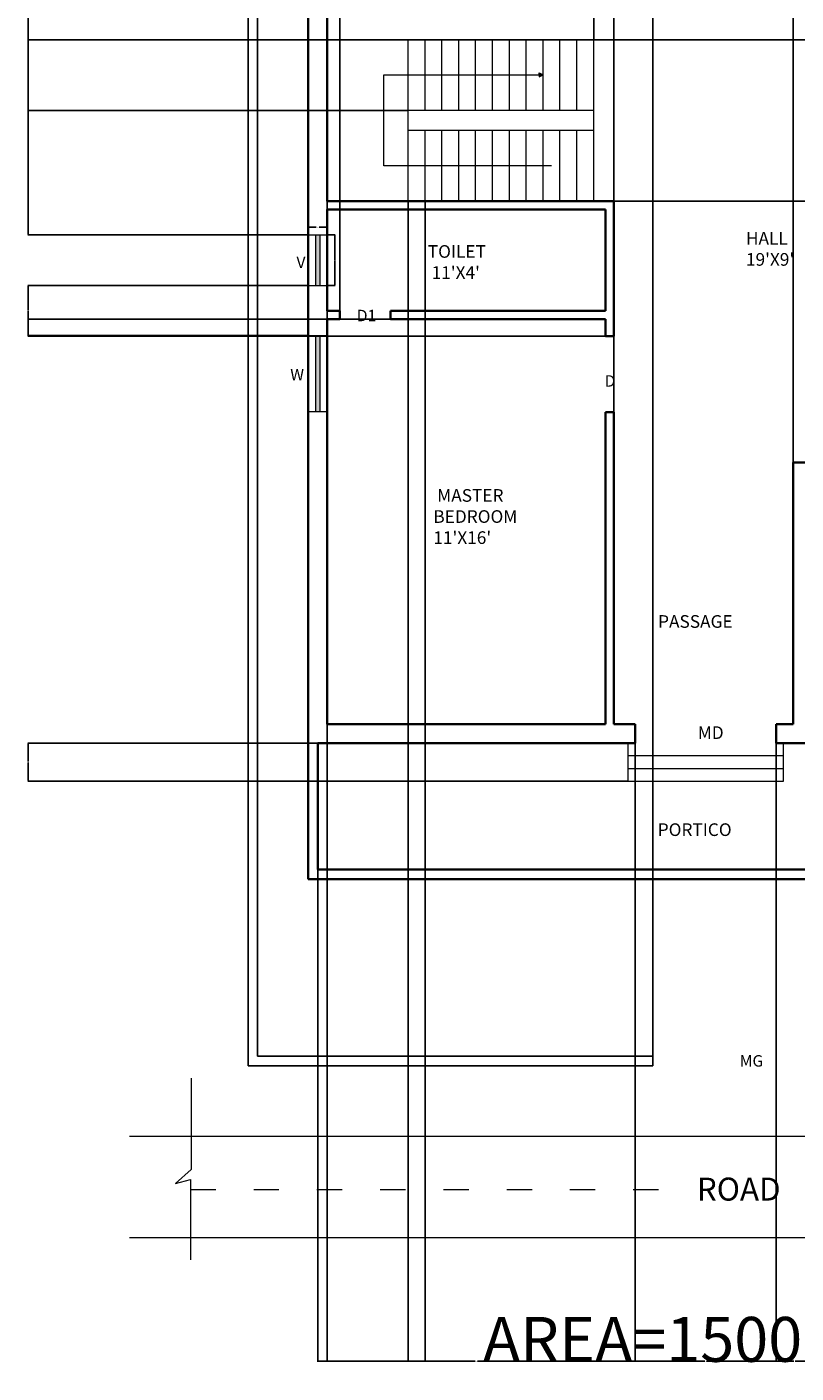
# Model space of a CAD drawing. Units: inches. Extents: x 502 to 1235, y -850 to 110.
# Tile 1 of 9: x 502 to 867, y -850 to -212. Entities that reach past the tile are written whole.
import ezdxf

# ---------------------------------------------------------------- set-up
doc = ezdxf.new("R2010")
doc.units = ezdxf.units.IN
doc.header["$MEASUREMENT"] = 0
doc.linetypes.add('ACAD_ISO03W100', pattern=[30, 12, -18])
for name, color, linetype, lineweight in [('A-ANNO-DIMS', 2, 'Continuous', 18), ('A-ANNO-SYMB', 1, 'Continuous', 13), ('A-ANNO-TEXT', 7, 'Continuous', 18), ('A-AREA-IDEN', 8, 'Continuous', 18), ('A-FLOR-STRS', 1, 'Continuous', 18), ('A-GLAZ-PATT', 5, 'Continuous', 13), ('C-PROP', 1, 'Continuous', 25), ('C-ROAD', 1, 'Continuous', 18), ('C-ROAD-CNTR', 1, 'ACAD_ISO03W100', 13), ('WALL', 1, 'Continuous', 35), ('WIN', 5, 'Continuous', 18)]:
    doc.layers.add(name, color=color, linetype=linetype, lineweight=lineweight)
doc.styles.get("Standard").update_dxf_attribs({"font": 'arial.ttf'})
doc.dimstyles.get("Standard").update_dxf_attribs({"dimtxt": 0.18, "dimasz": 0.18, "dimexe": 0.18, "dimexo": 0.0625, "dimgap": 0.09, "dimtad": 0, "dimtih": 1, "dimtoh": 1, "dimdec": 1, "dimzin": 0, "dimdsep": 46, "dimlunit": 4, "dimtxsty": 'Standard', "dimcen": 0.09, "dimadec": 0, "dimazin": 0, "dimtfac": 1, "dimtdec": 1, "dimtofl": 0, "dimtmove": 0, "dimatfit": 3, "dimfxl": 1, "dimtolj": 1, "dimtzin": 0, "dimarcsym": 0})

# ---------------------------------------------------------------- blocks, each defined once
blk = doc.blocks.new('WIN-36IN')
for p, q in [((0, 0), (0, 9)), ((36, 0), (36, 9)), ((0, 5.5), (36, 5.5)), ((0, 3.5), (36, 3.5))]:
    blk.add_line(p, q)
blk = doc.blocks.new('VENT-24IN')
for p, q in [((0, 0), (0, 9)), ((24, 0), (24, 9)), ((0, 5.5), (24, 5.5)), ((0, 3.5), (24, 3.5))]:
    blk.add_line(p, q)
blk = doc.blocks.new('*D16')
at = {"layer": 'A-ANNO-DIMS', "color": 0, "lineweight": -2, "transparency": 16777216}
for p, q in [((644.45, -310.35), (648.17, -310.35)), ((647.99, -310.53), (647.99, -322.16)), ((647.99, -334.17), (647.99, -322.53)), ((644.45, -334.35), (648.17, -334.35))]:
    blk.add_line(p, q, dxfattribs=at)
at = {"layer": 'A-ANNO-DIMS', "color": 0, "transparency": 16777216}
for points in [[(647.96, -310.53), (648.02, -310.53), (647.99, -310.35)], [(647.96, -334.17), (648.02, -334.17), (647.99, -334.35)]]:
    blk.add_solid(points, dxfattribs=at)
at = {"layer": 'Defpoints', "color": 0, "transparency": 16777216}
for p in [(644.39, -310.35), (644.39, -334.35), (647.99, -334.35)]:
    blk.add_point(p, dxfattribs=at)
at = {"layer": 'A-ANNO-DIMS', "color": 0, "transparency": 16777216, "insert": (647.99, -322.35), "char_height": 0.18, "attachment_point": 5}
blk.add_mtext('\\A1;VENT 2\'-0" TYP.', dxfattribs=at)
blk = doc.blocks.new('*D17')
at = {"layer": 'A-ANNO-DIMS', "color": 0, "lineweight": -2, "transparency": 16777216}
for p, q in [((635.39, -310.28), (635.39, -306.57)), ((635.57, -306.75), (639.25, -306.75)), ((644.21, -306.75), (640.53, -306.75)), ((644.39, -310.28), (644.39, -306.57))]:
    blk.add_line(p, q, dxfattribs=at)
at = {"layer": 'A-ANNO-DIMS', "color": 0, "transparency": 16777216}
for points in [[(635.57, -306.72), (635.57, -306.78), (635.39, -306.75)], [(644.21, -306.72), (644.21, -306.78), (644.39, -306.75)]]:
    blk.add_solid(points, dxfattribs=at)
at = {"layer": 'Defpoints', "color": 0, "transparency": 16777216}
for p in [(635.39, -310.35), (644.39, -306.75), (644.39, -310.35)]:
    blk.add_point(p, dxfattribs=at)
at = {"layer": 'A-ANNO-DIMS', "color": 0, "transparency": 16777216, "insert": (639.89, -306.75), "char_height": 0.18, "attachment_point": 5}
blk.add_mtext('\\A1;0\'-9" TYP.', dxfattribs=at)
blk = doc.blocks.new('*D25')
at = {"layer": 'A-ANNO-DIMS', "color": 0, "lineweight": -2, "transparency": 16777216}
for p, q in [((798.89, -699.78), (798.89, 63.98)), ((894.89, -699.78), (894.89, 63.98)), ((799.07, 63.8), (846.56, 63.8)), ((894.71, 63.8), (847.22, 63.8))]:
    blk.add_line(p, q, dxfattribs=at)
at = {"layer": 'A-ANNO-DIMS', "color": 0, "transparency": 16777216}
for points in [[(799.07, 63.83), (799.07, 63.77), (798.89, 63.8)], [(894.71, 63.83), (894.71, 63.77), (894.89, 63.8)]]:
    blk.add_solid(points, dxfattribs=at)
at = {"layer": 'Defpoints', "color": 0, "transparency": 16777216}
for p in [(894.89, 63.8), (798.89, -699.85), (894.89, -699.85)]:
    blk.add_point(p, dxfattribs=at)
at = {"layer": 'A-ANNO-DIMS', "color": 0, "transparency": 16777216, "insert": (846.89, 63.8), "char_height": 0.18, "attachment_point": 5}
blk.add_mtext('\\A1;8\'-0"', dxfattribs=at)
blk = doc.blocks.new('*D26')
at = {"layer": 'A-ANNO-DIMS', "color": 0, "lineweight": -2, "transparency": 16777216}
for p, q in [((606.89, -704.28), (606.89, 63.98)), ((798.89, -704.28), (798.89, 63.98)), ((607.07, 63.8), (702.5, 63.8)), ((798.71, 63.8), (703.28, 63.8))]:
    blk.add_line(p, q, dxfattribs=at)
at = {"layer": 'A-ANNO-DIMS', "color": 0, "transparency": 16777216}
for points in [[(607.07, 63.83), (607.07, 63.77), (606.89, 63.8)], [(798.71, 63.83), (798.71, 63.77), (798.89, 63.8)]]:
    blk.add_solid(points, dxfattribs=at)
at = {"layer": 'Defpoints', "color": 0, "transparency": 16777216}
for p in [(798.89, 63.8), (606.89, -704.35), (798.89, -704.35)]:
    blk.add_point(p, dxfattribs=at)
at = {"layer": 'A-ANNO-DIMS', "color": 0, "transparency": 16777216, "insert": (702.89, 63.8), "char_height": 0.18, "attachment_point": 5}
blk.add_mtext('\\A1;16\'-0"', dxfattribs=at)
blk = doc.blocks.new('*D27')
at = {"layer": 'A-ANNO-DIMS', "color": 0, "lineweight": -2, "transparency": 16777216}
for p, q in [((644.39, -217.78), (644.39, 63.98)), ((770.79, -217.78), (770.79, 63.98)), ((644.57, 63.8), (706.99, 63.8)), ((770.61, 63.8), (708.19, 63.8))]:
    blk.add_line(p, q, dxfattribs=at)
at = {"layer": 'A-ANNO-DIMS', "color": 0, "transparency": 16777216}
for points in [[(644.57, 63.83), (644.57, 63.77), (644.39, 63.8)], [(770.61, 63.83), (770.61, 63.77), (770.79, 63.8)]]:
    blk.add_solid(points, dxfattribs=at)
at = {"layer": 'Defpoints', "color": 0, "transparency": 16777216}
for p in [(770.79, 63.8), (644.39, -217.85), (770.79, -217.85)]:
    blk.add_point(p, dxfattribs=at)
at = {"layer": 'A-ANNO-DIMS', "color": 0, "transparency": 16777216, "insert": (707.59, 63.8), "char_height": 0.18, "attachment_point": 5}
blk.add_mtext('\\A1;10\'-6 1/2"', dxfattribs=at)
blk = doc.blocks.new('*D28')
at = {"layer": 'A-ANNO-DIMS', "color": 0, "lineweight": -2, "transparency": 16777216}
for p, q in [((770.85, -217.85), (1235.01, -217.85)), ((1234.83, -218.03), (1234.83, -255.91)), ((1234.83, -294.17), (1234.83, -256.28)), ((770.85, -294.35), (1235.01, -294.35))]:
    blk.add_line(p, q, dxfattribs=at)
at = {"layer": 'A-ANNO-DIMS', "color": 0, "transparency": 16777216}
for points in [[(1234.8, -218.03), (1234.86, -218.03), (1234.83, -217.85)], [(1234.8, -294.17), (1234.86, -294.17), (1234.83, -294.35)]]:
    blk.add_solid(points, dxfattribs=at)
at = {"layer": 'Defpoints', "color": 0, "transparency": 16777216}
for p in [(770.79, -217.85), (770.79, -294.35), (1234.83, -294.35)]:
    blk.add_point(p, dxfattribs=at)
at = {"layer": 'A-ANNO-DIMS', "color": 0, "transparency": 16777216, "insert": (1234.83, -256.1), "char_height": 0.18, "attachment_point": 5}
blk.add_mtext('\\A1;6\'-4 1/2"', dxfattribs=at)
blk = doc.blocks.new('*D29')
at = {"layer": 'A-ANNO-DIMS', "color": 0, "lineweight": -2, "transparency": 16777216}
for p, q in [((644.45, -193.85), (1235.01, -193.85)), ((1234.83, -194.03), (1234.83, -205.66)), ((1234.83, -217.67), (1234.83, -206.03)), ((644.45, -217.85), (1235.01, -217.85))]:
    blk.add_line(p, q, dxfattribs=at)
at = {"layer": 'A-ANNO-DIMS', "color": 0, "transparency": 16777216}
for points in [[(1234.8, -194.03), (1234.86, -194.03), (1234.83, -193.85)], [(1234.8, -217.67), (1234.86, -217.67), (1234.83, -217.85)]]:
    blk.add_solid(points, dxfattribs=at)
at = {"layer": 'Defpoints', "color": 0, "transparency": 16777216}
for p in [(644.39, -193.85), (644.39, -217.85), (1234.83, -217.85)]:
    blk.add_point(p, dxfattribs=at)
at = {"layer": 'A-ANNO-DIMS', "color": 0, "transparency": 16777216, "insert": (1234.83, -205.85), "char_height": 0.18, "attachment_point": 5}
blk.add_mtext('\\A1;2\'-0"', dxfattribs=at)
blk = doc.blocks.new('*D30')
at = {"layer": 'A-ANNO-DIMS', "color": 0, "lineweight": -2, "transparency": 16777216}
for p, q in [((644.39, -294.41), (644.39, -844.7)), ((682.79, -294.41), (682.79, -844.7)), ((644.57, -844.52), (663.05, -844.52)), ((682.61, -844.52), (664.13, -844.52))]:
    blk.add_line(p, q, dxfattribs=at)
at = {"layer": 'A-ANNO-DIMS', "color": 0, "transparency": 16777216}
for points in [[(644.57, -844.49), (644.57, -844.55), (644.39, -844.52)], [(682.61, -844.49), (682.61, -844.55), (682.79, -844.52)]]:
    blk.add_solid(points, dxfattribs=at)
at = {"layer": 'Defpoints', "color": 0, "transparency": 16777216}
for p in [(644.39, -294.35), (682.79, -294.35), (682.79, -844.52)]:
    blk.add_point(p, dxfattribs=at)
at = {"layer": 'A-ANNO-DIMS', "color": 0, "transparency": 16777216, "insert": (663.59, -844.52), "char_height": 0.18, "attachment_point": 5}
blk.add_mtext('\\A1;3\'-2 1/2"', dxfattribs=at)
blk = doc.blocks.new('*D31')
at = {"layer": 'A-ANNO-DIMS', "color": 0, "lineweight": -2, "transparency": 16777216}
for p, q in [((682.79, -294.41), (682.79, -844.7)), ((690.79, -294.41), (690.79, -844.7)), ((682.97, -844.52), (686.46, -844.52)), ((690.61, -844.52), (687.12, -844.52))]:
    blk.add_line(p, q, dxfattribs=at)
at = {"layer": 'A-ANNO-DIMS', "color": 0, "transparency": 16777216}
for points in [[(682.97, -844.49), (682.97, -844.55), (682.79, -844.52)], [(690.61, -844.49), (690.61, -844.55), (690.79, -844.52)]]:
    blk.add_solid(points, dxfattribs=at)
at = {"layer": 'Defpoints', "color": 0, "transparency": 16777216}
for p in [(682.79, -294.35), (690.79, -294.35), (690.79, -844.52)]:
    blk.add_point(p, dxfattribs=at)
at = {"layer": 'A-ANNO-DIMS', "color": 0, "transparency": 16777216, "insert": (686.79, -844.52), "char_height": 0.18, "attachment_point": 5}
blk.add_mtext('\\A1;0\'-8"', dxfattribs=at)
blk = doc.blocks.new('*D32')
at = {"layer": 'A-ANNO-DIMS', "color": 0, "lineweight": -2, "transparency": 16777216}
for p, q in [((682.73, -217.85), (502.37, -217.85)), ((502.55, -218.03), (502.55, -234.46)), ((502.55, -251.27), (502.55, -234.83)), ((682.73, -251.45), (502.37, -251.45))]:
    blk.add_line(p, q, dxfattribs=at)
at = {"layer": 'A-ANNO-DIMS', "color": 0, "transparency": 16777216}
for points in [[(502.52, -218.03), (502.58, -218.03), (502.55, -217.85)], [(502.52, -251.27), (502.58, -251.27), (502.55, -251.45)]]:
    blk.add_solid(points, dxfattribs=at)
at = {"layer": 'Defpoints', "color": 0, "transparency": 16777216}
for p in [(502.55, -217.85), (682.79, -217.85), (682.79, -251.45)]:
    blk.add_point(p, dxfattribs=at)
at = {"layer": 'A-ANNO-DIMS', "color": 0, "transparency": 16777216, "insert": (502.55, -234.65), "char_height": 0.18, "attachment_point": 5}
blk.add_mtext('\\A1;2\'-9 1/2"', dxfattribs=at)
blk = doc.blocks.new('*D39')
at = {"layer": 'A-ANNO-DIMS', "color": 0, "lineweight": -2, "transparency": 16777216}
for p, q in [((644.39, -346.28), (644.39, 63.98)), ((650.39, -346.28), (650.39, 63.98)), ((644.57, 63.8), (647.06, 63.8)), ((650.21, 63.8), (647.72, 63.8))]:
    blk.add_line(p, q, dxfattribs=at)
at = {"layer": 'A-ANNO-DIMS', "color": 0, "transparency": 16777216}
for points in [[(644.57, 63.83), (644.57, 63.77), (644.39, 63.8)], [(650.21, 63.83), (650.21, 63.77), (650.39, 63.8)]]:
    blk.add_solid(points, dxfattribs=at)
at = {"layer": 'Defpoints', "color": 0, "transparency": 16777216}
for p in [(650.39, 63.8), (644.39, -346.35), (650.39, -346.35)]:
    blk.add_point(p, dxfattribs=at)
at = {"layer": 'A-ANNO-DIMS', "color": 0, "transparency": 16777216, "insert": (647.39, 63.8), "char_height": 0.18, "attachment_point": 5}
blk.add_mtext('\\A1;0\'-6"', dxfattribs=at)
blk = doc.blocks.new('*D40')
at = {"layer": 'A-ANNO-DIMS', "color": 0, "lineweight": -2, "transparency": 16777216}
for p, q in [((776.33, -350.35), (502.37, -350.35)), ((502.55, -350.53), (502.55, -354.16)), ((502.55, -358.17), (502.55, -354.53)), ((776.33, -358.35), (502.37, -358.35))]:
    blk.add_line(p, q, dxfattribs=at)
at = {"layer": 'A-ANNO-DIMS', "color": 0, "transparency": 16777216}
for points in [[(502.52, -350.53), (502.58, -350.53), (502.55, -350.35)], [(502.52, -358.17), (502.58, -358.17), (502.55, -358.35)]]:
    blk.add_solid(points, dxfattribs=at)
at = {"layer": 'Defpoints', "color": 0, "transparency": 16777216}
for p in [(776.39, -350.35), (502.55, -358.35), (776.39, -358.35)]:
    blk.add_point(p, dxfattribs=at)
at = {"layer": 'A-ANNO-DIMS', "color": 0, "transparency": 16777216, "insert": (502.55, -354.35), "char_height": 0.18, "attachment_point": 5}
blk.add_mtext('\\A1;0\'-8"', dxfattribs=at)
blk = doc.blocks.new('*D44')
at = {"layer": 'A-ANNO-DIMS', "color": 0, "lineweight": -2, "transparency": 16777216}
for p, q in [((780.39, -542.28), (780.39, 63.98)), ((865.39, -542.28), (865.39, 63.98)), ((780.57, 63.8), (822.56, 63.8)), ((865.21, 63.8), (823.22, 63.8))]:
    blk.add_line(p, q, dxfattribs=at)
at = {"layer": 'A-ANNO-DIMS', "color": 0, "transparency": 16777216}
for points in [[(780.57, 63.83), (780.57, 63.77), (780.39, 63.8)], [(865.21, 63.83), (865.21, 63.77), (865.39, 63.8)]]:
    blk.add_solid(points, dxfattribs=at)
at = {"layer": 'Defpoints', "color": 0, "transparency": 16777216}
for p in [(865.39, 63.8), (780.39, -542.35), (865.39, -542.35)]:
    blk.add_point(p, dxfattribs=at)
at = {"layer": 'A-ANNO-DIMS', "color": 0, "transparency": 16777216, "insert": (822.89, 63.8), "char_height": 0.18, "attachment_point": 5}
blk.add_mtext('\\A1;7\'-1"', dxfattribs=at)
blk = doc.blocks.new('*D45')
at = {"layer": 'A-ANNO-DIMS', "color": 0, "lineweight": -2, "transparency": 16777216}
for p, q in [((790.39, -551.41), (790.39, -844.7)), ((857.39, -551.41), (857.39, -844.7)), ((790.57, -844.52), (823.56, -844.52)), ((857.21, -844.52), (824.22, -844.52))]:
    blk.add_line(p, q, dxfattribs=at)
at = {"layer": 'A-ANNO-DIMS', "color": 0, "transparency": 16777216}
for points in [[(790.57, -844.49), (790.57, -844.55), (790.39, -844.52)], [(857.21, -844.49), (857.21, -844.55), (857.39, -844.52)]]:
    blk.add_solid(points, dxfattribs=at)
at = {"layer": 'Defpoints', "color": 0, "transparency": 16777216}
for p in [(790.39, -551.35), (857.39, -551.35), (857.39, -844.52)]:
    blk.add_point(p, dxfattribs=at)
at = {"layer": 'A-ANNO-DIMS', "color": 0, "transparency": 16777216, "insert": (823.89, -844.52), "char_height": 0.18, "attachment_point": 5}
blk.add_mtext('\\A1;5\'-7"', dxfattribs=at)
blk = doc.blocks.new('*D46')
at = {"layer": 'A-ANNO-DIMS', "color": 0, "lineweight": -2, "transparency": 16777216}
for p, q in [((639.89, -551.41), (639.89, -844.7)), ((790.39, -551.41), (790.39, -844.7)), ((640.07, -844.52), (714.54, -844.52)), ((790.21, -844.52), (715.74, -844.52))]:
    blk.add_line(p, q, dxfattribs=at)
at = {"layer": 'A-ANNO-DIMS', "color": 0, "transparency": 16777216}
for points in [[(640.07, -844.49), (640.07, -844.55), (639.89, -844.52)], [(790.21, -844.49), (790.21, -844.55), (790.39, -844.52)]]:
    blk.add_solid(points, dxfattribs=at)
at = {"layer": 'Defpoints', "color": 0, "transparency": 16777216}
for p in [(639.89, -551.35), (790.39, -551.35), (790.39, -844.52)]:
    blk.add_point(p, dxfattribs=at)
at = {"layer": 'A-ANNO-DIMS', "color": 0, "transparency": 16777216, "insert": (715.14, -844.52), "char_height": 0.18, "attachment_point": 5}
blk.add_mtext('\\A1;12\'-6 1/2"', dxfattribs=at)
blk = doc.blocks.new('*D47')
at = {"layer": 'A-ANNO-DIMS', "color": 0, "lineweight": -2, "transparency": 16777216}
for p, q in [((857.39, -551.41), (857.39, -844.7)), ((874.64, -551.41), (874.64, -844.7)), ((857.57, -844.52), (865.69, -844.52)), ((874.46, -844.52), (866.34, -844.52))]:
    blk.add_line(p, q, dxfattribs=at)
at = {"layer": 'A-ANNO-DIMS', "color": 0, "transparency": 16777216}
for points in [[(857.57, -844.49), (857.57, -844.55), (857.39, -844.52)], [(874.46, -844.49), (874.46, -844.55), (874.64, -844.52)]]:
    blk.add_solid(points, dxfattribs=at)
at = {"layer": 'Defpoints', "color": 0, "transparency": 16777216}
for p in [(857.39, -551.35), (874.64, -551.35), (874.64, -844.52)]:
    blk.add_point(p, dxfattribs=at)
at = {"layer": 'A-ANNO-DIMS', "color": 0, "transparency": 16777216, "insert": (866.01, -844.52), "char_height": 0.18, "attachment_point": 5}
blk.add_mtext('\\A1;1\'-5"', dxfattribs=at)
blk = doc.blocks.new('*D48')
at = {"layer": 'A-ANNO-DIMS', "color": 0, "lineweight": -2, "transparency": 16777216}
for p, q in [((786.88, -551.35), (502.37, -551.35)), ((502.55, -551.53), (502.55, -560.16)), ((502.55, -569.17), (502.55, -560.53)), ((786.88, -569.35), (502.37, -569.35))]:
    blk.add_line(p, q, dxfattribs=at)
at = {"layer": 'A-ANNO-DIMS', "color": 0, "transparency": 16777216}
for points in [[(502.52, -551.53), (502.58, -551.53), (502.55, -551.35)], [(502.52, -569.17), (502.58, -569.17), (502.55, -569.35)]]:
    blk.add_solid(points, dxfattribs=at)
at = {"layer": 'Defpoints', "color": 0, "transparency": 16777216}
for p in [(502.55, -551.35), (786.94, -551.35), (786.94, -569.35)]:
    blk.add_point(p, dxfattribs=at)
at = {"layer": 'A-ANNO-DIMS', "color": 0, "transparency": 16777216, "insert": (502.55, -560.35), "char_height": 0.18, "attachment_point": 5}
blk.add_mtext('\\A1;1\'-6"', dxfattribs=at)
blk = doc.blocks.new('*D52')
at = {"layer": 'A-ANNO-DIMS', "color": 0, "lineweight": -2, "transparency": 16777216}
for p, q in [((635.33, -60.85), (502.37, -60.85)), ((502.55, -61.03), (502.55, -185.41)), ((502.55, -310.17), (502.55, -185.78)), ((635.33, -310.35), (502.37, -310.35))]:
    blk.add_line(p, q, dxfattribs=at)
at = {"layer": 'A-ANNO-DIMS', "color": 0, "transparency": 16777216}
for points in [[(502.52, -61.03), (502.58, -61.03), (502.55, -60.85)], [(502.52, -310.17), (502.58, -310.17), (502.55, -310.35)]]:
    blk.add_solid(points, dxfattribs=at)
at = {"layer": 'Defpoints', "color": 0, "transparency": 16777216}
for p in [(502.55, -60.85), (635.39, -60.85), (635.39, -310.35)]:
    blk.add_point(p, dxfattribs=at)
at = {"layer": 'A-ANNO-DIMS', "color": 0, "transparency": 16777216, "insert": (502.55, -185.6), "char_height": 0.18, "attachment_point": 5}
blk.add_mtext('\\A1;20\'-9 1/2"', dxfattribs=at)
blk = doc.blocks.new('*D53')
at = {"layer": 'A-ANNO-DIMS', "color": 0, "lineweight": -2, "transparency": 16777216}
for p, q in [((635.33, -334.35), (502.37, -334.35)), ((502.55, -334.53), (502.55, -346.02)), ((502.55, -357.88), (502.55, -346.38)), ((635.33, -358.06), (502.37, -358.06))]:
    blk.add_line(p, q, dxfattribs=at)
at = {"layer": 'A-ANNO-DIMS', "color": 0, "transparency": 16777216}
for points in [[(502.52, -334.53), (502.58, -334.53), (502.55, -334.35)], [(502.52, -357.88), (502.58, -357.88), (502.55, -358.06)]]:
    blk.add_solid(points, dxfattribs=at)
at = {"layer": 'Defpoints', "color": 0, "transparency": 16777216}
for p in [(635.39, -334.35), (502.55, -358.06), (635.39, -358.06)]:
    blk.add_point(p, dxfattribs=at)
at = {"layer": 'A-ANNO-DIMS', "color": 0, "transparency": 16777216, "insert": (502.55, -346.2), "char_height": 0.18, "attachment_point": 5}
blk.add_mtext('\\A1;1\'-11 1/2"', dxfattribs=at)

msp = doc.modelspace()

# ---------------------------------------------------------------- hatches: boundary and pattern name
at = {"layer": 'A-ANNO-SYMB'}
h = msp.add_hatch(color=256, dxfattribs=at)
h.dxf.hatch_style = 1
h.paths.add_polyline_path([(746.79, -234.44), (744.91, -233.44), (744.91, -234.44), (744.91, -235.44)])
at = {"layer": 'A-GLAZ-PATT'}
h = msp.add_hatch(color=256, dxfattribs=at)
h.dxf.hatch_style = 1
h.paths.add_polyline_path([(769.5, -64.35), (769.5, -66.35), (805.5, -66.35), (805.5, -64.35)])
h.paths.add_polyline_path([(845.65, -64.35), (821.65, -64.35), (821.65, -66.35), (845.65, -66.35)])
h.paths.add_polyline_path([(995.07, -64.35), (959.07, -64.35), (959.07, -66.35), (995.07, -66.35)])
h.paths.add_polyline_path([(1006.89, -358.85), (1004.89, -358.85), (1004.89, -394.85), (1006.89, -394.85)])
h.paths.add_polyline_path([(1006.89, -435.74), (1004.89, -435.74), (1004.89, -471.74), (1006.89, -471.74)])
h.paths.add_polyline_path([(874.64, -545.85), (874.64, -547.85), (910.64, -547.85), (910.64, -545.85)])
h.paths.add_polyline_path([(640.89, -310.35), (638.89, -310.35), (638.89, -334.35), (640.89, -334.35)])
h.paths.add_polyline_path([(640.89, -358.06), (638.89, -358.06), (638.89, -394.06), (640.89, -394.06)])

# ---------------------------------------------------------------- linework, layer by layer
at = {"layer": 'A-ANNO-SYMB'}
for p, q in [((671.31, -277.65), (671.31, -234.44)), ((671.31, -234.44), (743.02, -234.44)), ((743.02, -234.44), (744.91, -234.44)), ((744.91, -234.44), (744.91, -233.44)), ((744.91, -233.44), (746.79, -234.44)), ((744.91, -234.44), (744.91, -235.44)), ((744.91, -235.44), (746.79, -234.44)), ((750.76, -277.65), (671.31, -277.65)), ((579.9, -710.31), (579.9, -753.61)), ((579.9, -753.61), (572.43, -760.17)), ((572.43, -760.17), (579.54, -758.33)), ((579.54, -758.33), (579.54, -796.37))]:
    msp.add_line(p, q, dxfattribs=at)
at = {"layer": 'A-FLOR-STRS'}
for p, q in [((770.79, -217.85), (644.39, -217.85)), ((682.79, -251.45), (682.79, -217.85)), ((690.79, -251.45), (690.79, -217.85)), ((698.79, -251.45), (698.79, -217.85)), ((706.79, -251.45), (706.79, -217.85)), ((714.79, -251.45), (714.79, -217.85)), ((722.79, -251.45), (722.79, -217.85)), ((730.79, -251.45), (730.79, -217.85)), ((738.79, -251.45), (738.79, -217.85)), ((746.79, -251.45), (746.79, -217.85)), ((754.79, -251.45), (754.79, -217.85)), ((762.79, -251.45), (762.79, -217.85)), ((770.79, -251.45), (770.79, -217.85)), ((682.79, -294.35), (682.79, -251.45)), ((770.79, -251.45), (682.79, -251.45)), ((770.79, -294.35), (770.79, -251.45)), ((682.79, -260.75), (770.79, -260.75)), ((690.79, -294.35), (690.79, -260.75)), ((698.79, -294.35), (698.79, -260.75)), ((706.79, -294.35), (706.79, -260.75)), ((714.79, -294.35), (714.79, -260.75)), ((722.79, -294.35), (722.79, -260.75)), ((730.79, -294.35), (730.79, -260.75)), ((738.79, -294.35), (738.79, -260.75)), ((746.79, -294.35), (746.79, -260.75)), ((754.79, -294.35), (754.79, -260.75)), ((762.79, -294.35), (762.79, -260.75)), ((786.94, -551.35), (786.94, -569.35)), ((860.86, -569.35), (860.86, -551.35)), ((860.86, -557.35), (786.94, -557.35)), ((786.94, -563.35), (860.86, -563.35)), ((786.94, -569.35), (860.86, -569.35))]:
    msp.add_line(p, q, dxfattribs=at)
at = {"layer": 'C-PROP'}
for p, q in [((606.89, -704.35), (606.89, 15.65)), ((611.39, -699.85), (611.39, 11.15)), ((611.39, -699.85), (798.89, -699.85)), ((798.89, -704.35), (798.89, -699.85)), ((606.89, -704.35), (798.89, -704.35))]:
    msp.add_line(p, q, dxfattribs=at)
at = {"layer": 'C-ROAD'}
for p, q in [((550.7, -737.83), (1186.68, -737.83)), ((550.7, -785.83), (1186.68, -785.83))]:
    msp.add_line(p, q, dxfattribs=at)
at = {"layer": 'C-ROAD-CNTR'}
msp.add_line((579.54, -763.02), (816.08, -763.02), dxfattribs=at)
at = {"layer": 'WALL'}
for p, q in [((635.39, -615.85), (635.39, -60.85)), ((644.39, -294.35), (644.39, -193.85)), ((644.39, -294.35), (780.39, -294.35)), ((644.39, -298.35), (776.39, -298.35)), ((644.39, -346.35), (644.39, -298.35)), ((776.39, -346.35), (776.39, -298.35)), ((780.39, -358.35), (780.39, -294.35)), ((644.39, -346.35), (650.39, -346.35)), ((644.39, -350.35), (650.39, -350.35)), ((644.39, -542.35), (644.39, -350.35)), ((650.39, -350.35), (650.39, -346.35)), ((674.39, -350.35), (674.39, -346.35)), ((674.39, -346.35), (776.39, -346.35)), ((674.39, -350.35), (776.39, -350.35)), ((776.39, -358.35), (776.39, -350.35)), ((776.39, -358.35), (780.39, -358.35)), ((776.39, -542.35), (776.39, -394.35)), ((776.39, -394.35), (780.39, -394.35)), ((780.39, -542.35), (780.39, -394.35)), ((865.39, -542.35), (865.39, -418.35)), ((865.39, -418.35), (877.39, -418.35)), ((644.39, -542.35), (776.39, -542.35)), ((780.39, -542.35), (790.39, -542.35)), ((790.39, -551.35), (790.39, -542.35)), ((857.39, -551.35), (857.39, -542.35)), ((857.39, -542.35), (865.39, -542.35)), ((639.89, -551.35), (790.39, -551.35)), ((639.89, -611.35), (639.89, -551.35)), ((857.39, -551.35), (1005.89, -551.35)), ((639.89, -611.35), (1005.89, -611.35)), ((635.39, -615.85), (1010.39, -615.85))]:
    msp.add_line(p, q, dxfattribs=at)

# ---------------------------------------------------------------- block references
at = {"layer": 'WIN'}
for name, p, rotation in [('VENT-24IN', (635.39, -310.35), 269.9999999999994), ('WIN-36IN', (635.39, -358.06), 270.0000000000004)]:
    msp.add_blockref(name, p, dxfattribs=dict(at, rotation=rotation))

# ---------------------------------------------------------------- texts
at = {"layer": 'A-ANNO-TEXT'}
for s, height, p in [('V', 5.44, (629.83, -326.1)), ('D1', 5.444, (658.43, -351.34)), ('W', 5.44, (626.89, -379.36)), ('D', 5.44, (775.99, -382.35)), ('MD', 6, (820.15, -549.4)), ('MG', 5.444, (840.05, -704.78))]:
    msp.add_text(s, height=height, dxfattribs=at).set_placement(p)
at = {"layer": 'A-ANNO-TEXT', "insert": (819.71, -757.43), "char_height": 10.889, "attachment_point": 1}
msp.add_mtext_dynamic_manual_height_columns('ROAD', width=44.8037, gutter_width=1.81, heights=[0], dxfattribs=at)
at = {"layer": 'A-AREA-IDEN', "attachment_point": 1}
for s, width, gutter_width, insert, char_height in [("HALL     19'X9'", 24.7419, 1, (843, -308.99), 6), ("   TOILET\\P    11'X4'", 39.4484, 1, (686.61, -315.23), 6), (" MASTER     BEDROOM\\P11'X16'", 44.6743, 1, (694.75, -430.92), 6), ('  PASSAGE', 53.3957, 1, (797.65, -490.69), 6), ('PORTICO', 39.567, 1, (801.16, -589.41), 6), ('AREA=1500 SQFT', 263.9184, 3.55, (718.27, -823.48), 21.2807)]:
    msp.add_mtext_dynamic_manual_height_columns(s, width=width, gutter_width=gutter_width, heights=[0], dxfattribs=dict(at, insert=insert, char_height=char_height))

# ---------------------------------------------------------------- dimensions: what is measured, and where the dimension line sits
at = {"layer": 'A-ANNO-DIMS'}
for base, p1, p2, picture, middle in [((798.89, 63.8), (606.89, -704.35), (798.89, -704.35), '*D26', (702.89, 63.8)), ((770.79, 63.8), (644.39, -217.85), (770.79, -217.85), '*D27', (707.59, 63.8)), ((650.39, 63.8), (644.39, -346.35), (650.39, -346.35), '*D39', (647.39, 63.8)), ((865.39, 63.8), (780.39, -542.35), (865.39, -542.35), '*D44', (822.89, 63.8)), ((894.89, 63.8), (798.89, -699.85), (894.89, -699.85), '*D25', (846.89, 63.8)), ((682.79, -844.52), (644.39, -294.35), (682.79, -294.35), '*D30', (663.59, -844.52)), ((690.79, -844.52), (682.79, -294.35), (690.79, -294.35), '*D31', (686.79, -844.52)), ((790.39, -844.52), (639.89, -551.35), (790.39, -551.35), '*D46', (715.14, -844.52)), ((857.39, -844.52), (790.39, -551.35), (857.39, -551.35), '*D45', (823.89, -844.52)), ((874.6386, -844.5172), (857.3902, -551.3456), (874.6386, -551.3456), '*D47', (866.0144, -844.5172))]:
    dim = msp.add_linear_dim(base=base, p1=p1, p2=p2, dimstyle='Standard', override={"dimdec": 1, "dimlfac": 1, "dimrnd": 0, "dimzin": 1, "dimdsep": 46, "dimlunit": 4, "dimfrac": 2}, dxfattribs=at)
    dim.commit()
    dim.dimension.update_dxf_attribs({"geometry": picture, "text_midpoint": middle})
for base, p1, p2, picture, middle in [((502.55, -60.85), (635.39, -310.35), (635.39, -60.85), '*D52', (502.55, -185.6)), ((1234.83, -217.85), (644.39, -193.85), (644.39, -217.85), '*D29', (1234.83, -205.85)), ((502.55, -217.85), (682.79, -251.45), (682.79, -217.85), '*D32', (502.55, -234.65)), ((1234.83, -294.35), (770.79, -217.85), (770.79, -294.35), '*D28', (1234.83, -256.1)), ((502.55, -358.06), (635.39, -334.35), (635.39, -358.06), '*D53', (502.55, -346.2)), ((502.55, -358.35), (776.39, -350.35), (776.39, -358.35), '*D40', (502.55, -354.35)), ((502.55, -551.35), (786.94, -569.35), (786.94, -551.35), '*D48', (502.55, -560.35))]:
    dim = msp.add_linear_dim(base=base, p1=p1, p2=p2, angle=90, dimstyle='Standard', override={"dimdec": 1, "dimlfac": 1, "dimrnd": 0, "dimzin": 1, "dimdsep": 46, "dimlunit": 4, "dimfrac": 2}, dxfattribs=at)
    dim.commit()
    dim.dimension.update_dxf_attribs({"geometry": picture, "text_midpoint": middle})
dim = msp.add_linear_dim(base=(644.39, -306.75), p1=(635.39, -310.35), p2=(644.39, -310.35), text='<> TYP.', dimstyle='Standard', override={"dimdec": 1, "dimlfac": 1, "dimrnd": 0, "dimzin": 1, "dimdsep": 46, "dimlunit": 4, "dimfrac": 2}, dxfattribs=at)
dim.commit()
dim.dimension.update_dxf_attribs({"geometry": '*D17', "text_midpoint": (639.89, -306.75)})
dim = msp.add_linear_dim(base=(647.99, -334.35), p1=(644.39, -310.35), p2=(644.39, -334.35), angle=270, text='VENT <> TYP.', dimstyle='Standard', override={"dimdec": 1, "dimlfac": 1, "dimrnd": 0, "dimzin": 1, "dimdsep": 46, "dimlunit": 4, "dimfrac": 2}, dxfattribs=at)
dim.commit()
dim.dimension.update_dxf_attribs({"geometry": '*D16', "text_midpoint": (647.99, -322.35)})

doc.saveas('drawing.dxf')
